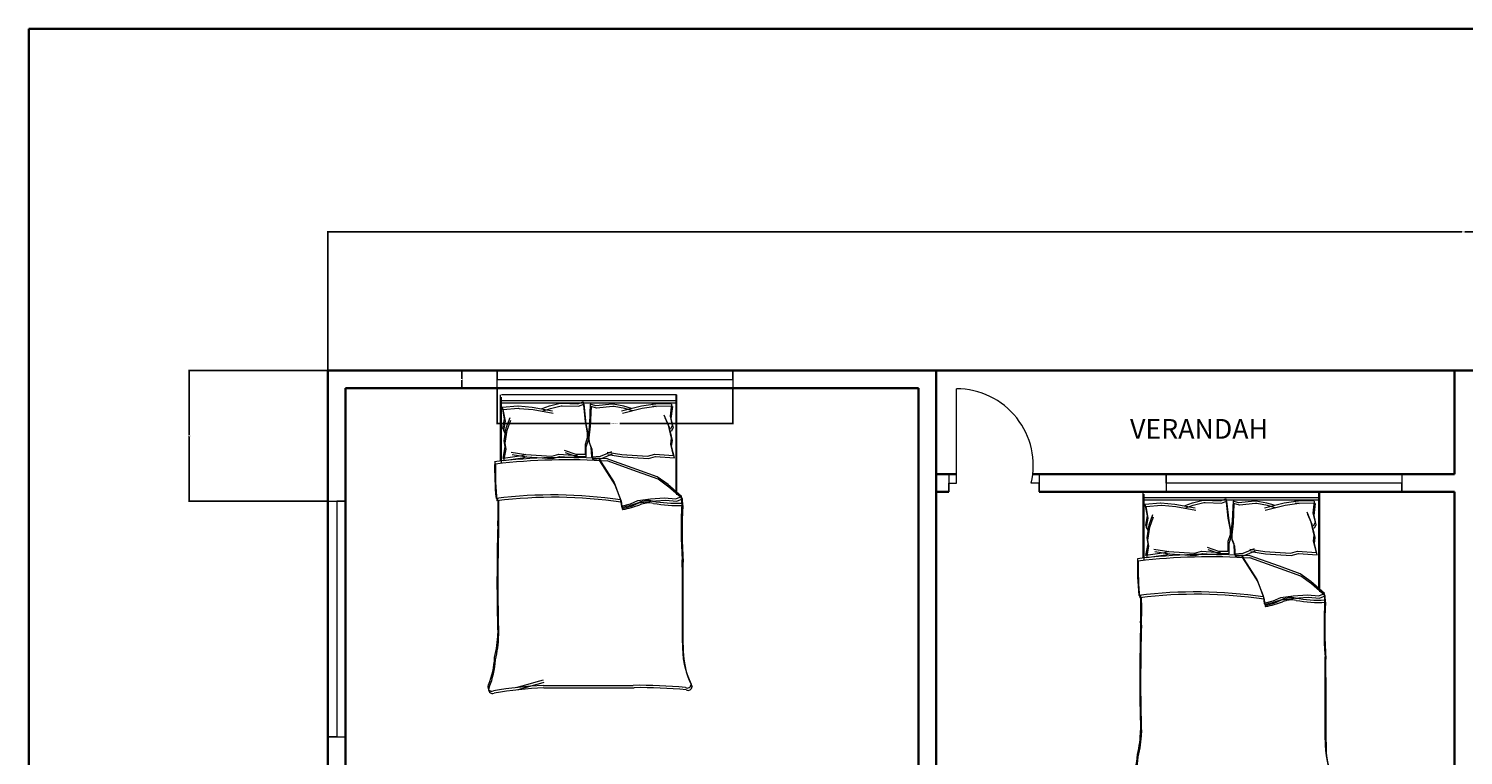
# Model space of a CAD drawing. Units: inches. Extents: x 2234 to 3001, y 1541 to 2386.
# Tile 7 of 12: x 2234 to 2599, y 2201 to 2386. Entities that reach past the tile are written whole.
import ezdxf

# ---------------------------------------------------------------- set-up
doc = ezdxf.new("R2010")
doc.units = ezdxf.units.IN
for name, color, linetype, lineweight in [('A-ANNO-DIMS', 2, 'Continuous', 18), ('A-ANNO-TTLB', 7, 'Continuous', 35), ('A-AREA-IDEN', 7, 'Continuous', 18), ('A-DOOR', 3, 'Continuous', 18), ('A-FURN', 9, 'Continuous', 13), ('A-GLAZ', 4, 'Continuous', 18), ('A-WALL', 7, 'Continuous', 35)]:
    doc.layers.add(name, color=color, linetype=linetype, lineweight=lineweight)
doc.styles.get("Standard").update_dxf_attribs({"font": 'arial.ttf'})
doc.dimstyles.get("Standard").update_dxf_attribs({"dimtxt": 0.18, "dimasz": 0.18, "dimexe": 0.18, "dimexo": 0.0625, "dimgap": 0.09, "dimtad": 0, "dimtih": 1, "dimtoh": 1, "dimdec": 4, "dimzin": 0, "dimdsep": 46, "dimtxsty": 'Standard', "dimcen": 0.09, "dimadec": 0, "dimazin": 0, "dimtfac": 1, "dimtdec": 4, "dimtofl": 0, "dimtmove": 0, "dimatfit": 3, "dimfxl": 1, "dimtolj": 1, "dimtzin": 0, "dimarcsym": 0})

# ---------------------------------------------------------------- blocks, each defined once
blk = doc.blocks.new('WIN-60-A')
for p, q in [((0, 60), (4.5, 60)), ((4.5, 60), (2.25, 60)), ((2.25, 60), (2.25, 0)), ((2.25, 0), (0, 0)), ((0, 0), (4.5, 0))]:
    blk.add_line(p, q)
blk = doc.blocks.new('WIN-60-B')
for p, q in [((0, 60), (4.5, 60)), ((4.5, 60), (2.25, 60)), ((2.25, 60), (2.25, 0)), ((4.5, 0), (0, 0)), ((2.25, 0), (4.5, 0))]:
    blk.add_line(p, q)
blk = doc.blocks.new('BED-DOUBLE-A')
for p, q in [((3.24, 59.14), (3.24, 76.05)), ((3.24, 59.14), (3.24, 76.05)), ((3.24, 74.62), (47.87, 74.62)), ((3.24, 74.62), (47.87, 74.62)), ((48.08, 76.05), (3.46, 76.05)), ((3.46, 58.54), (3.46, 75.45)), ((3.46, 58.54), (3.46, 75.45)), ((3.46, 74.02), (48.08, 74.02)), ((3.46, 74.02), (48.08, 74.02)), ((3.64, 72.93), (7.64, 73.24)), ((3.64, 72.93), (7.64, 73.24)), ((7.64, 73.24), (7.74, 73.22)), ((7.64, 73.24), (7.74, 73.22)), ((7.74, 73.22), (11.31, 72.95)), ((7.74, 73.22), (11.31, 72.95)), ((13.87, 72.55), (15.76, 73.22)), ((13.87, 72.55), (15.76, 73.22)), ((15.76, 73.22), (18.46, 73.9)), ((15.76, 73.22), (18.46, 73.9)), ((15.97, 72.62), (18.67, 73.3)), ((15.97, 72.62), (18.67, 73.3)), ((18.46, 73.9), (18.76, 73.9)), ((18.46, 73.9), (18.76, 73.9)), ((18.67, 73.3), (18.97, 73.3)), ((18.67, 73.3), (18.97, 73.3)), ((18.76, 73.9), (22.91, 73.76)), ((18.76, 73.9), (22.91, 73.76)), ((18.97, 73.3), (23.12, 73.16)), ((18.97, 73.3), (23.12, 73.16)), ((22.91, 73.76), (24.26, 74.3)), ((22.91, 73.76), (24.26, 74.3)), ((23.12, 73.16), (24.47, 73.7)), ((23.12, 73.16), (24.47, 73.7)), ((24.26, 74.3), (24.8, 69.31)), ((24.26, 74.3), (24.8, 69.31)), ((24.47, 73.7), (25.01, 68.71)), ((24.47, 73.7), (25.01, 68.71)), ((26.12, 73.72), (25.9, 68.7)), ((26.12, 73.72), (25.9, 68.7)), ((26.34, 73.12), (26.11, 68.1)), ((26.34, 73.12), (26.11, 68.1)), ((27.5, 73.27), (26.12, 73.72)), ((27.5, 73.27), (26.12, 73.72)), ((27.72, 72.67), (26.34, 73.12)), ((27.72, 72.67), (26.34, 73.12)), ((31.64, 73.66), (27.5, 73.27)), ((31.64, 73.66), (27.5, 73.27)), ((31.94, 73.68), (31.64, 73.66)), ((31.94, 73.68), (31.64, 73.66)), ((34.67, 73.17), (31.94, 73.68)), ((34.67, 73.17), (31.94, 73.68)), ((39.14, 73.18), (34.08, 71.92)), ((39.14, 73.18), (34.08, 71.92)), ((36.6, 72.62), (34.67, 73.17)), ((36.6, 72.62), (34.67, 73.17)), ((42.68, 73.67), (39.14, 73.18)), ((42.68, 73.67), (39.14, 73.18)), ((46.79, 73.66), (41.75, 73.75)), ((41.75, 73.75), (42.68, 73.67)), ((46.79, 73.66), (41.75, 73.75)), ((41.75, 73.75), (42.68, 73.67)), ((47.01, 73.06), (41.96, 73.15)), ((41.96, 73.15), (42.9, 73.08)), ((47, 73.06), (41.96, 73.15)), ((41.96, 73.15), (42.9, 73.08)), ((46.79, 73.66), (46.44, 70.66)), ((46.79, 73.66), (46.44, 70.66)), ((47.87, 76.05), (47.87, 51.2)), ((47.87, 76.05), (47.87, 51.2)), ((48.08, 76.05), (48.08, 75.45)), ((48.08, 75.45), (48.08, 50.6)), ((48.08, 75.45), (48.08, 50.6)), ((3.64, 72.95), (4.18, 69.98)), ((3.64, 72.95), (4.18, 69.98)), ((4.18, 69.98), (3.77, 67.55)), ((4.18, 69.98), (3.77, 67.55)), ((3.85, 72.33), (7.85, 72.64)), ((3.85, 72.33), (7.85, 72.64)), ((3.85, 72.35), (4.39, 69.38)), ((3.85, 72.35), (4.39, 69.38)), ((4.72, 67.69), (5.66, 70.25)), ((4.72, 67.69), (5.66, 70.25)), ((4.93, 67.09), (5.87, 69.65)), ((4.93, 67.09), (5.87, 69.65)), ((7.85, 72.64), (7.95, 72.62)), ((7.85, 72.64), (7.95, 72.62)), ((7.95, 72.62), (11.52, 72.35)), ((7.95, 72.62), (11.52, 72.35)), ((11.31, 72.95), (16.44, 72.01)), ((11.31, 72.95), (16.44, 72.01)), ((11.52, 72.35), (16.65, 71.41)), ((11.52, 72.35), (16.65, 71.41)), ((14.08, 71.95), (15.97, 72.62)), ((14.08, 71.95), (15.97, 72.62)), ((31.85, 73.06), (27.72, 72.67)), ((31.85, 73.06), (27.72, 72.67)), ((32.15, 73.08), (31.85, 73.06)), ((32.15, 73.08), (31.85, 73.06)), ((34.89, 72.58), (32.15, 73.08)), ((34.89, 72.58), (32.15, 73.08)), ((39.35, 72.58), (34.29, 71.32)), ((39.35, 72.58), (34.29, 71.32)), ((36.82, 72.02), (34.89, 72.58)), ((36.82, 72.02), (34.89, 72.58)), ((42.9, 73.08), (39.35, 72.58)), ((42.9, 73.08), (39.35, 72.58)), ((46.04, 68.34), (44.94, 70.84)), ((46.04, 68.34), (44.94, 70.84)), ((46.26, 67.74), (45.15, 70.24)), ((46.26, 67.74), (45.15, 70.24)), ((46.44, 70.66), (46.99, 68.26)), ((46.44, 70.66), (46.99, 68.26)), ((47.01, 73.06), (46.65, 70.07)), ((47, 73.06), (46.65, 70.07)), ((46.65, 70.07), (47.21, 67.66)), ((46.65, 70.07), (47.21, 67.66)), ((3.77, 67.55), (4.31, 66.61)), ((3.77, 67.55), (4.31, 66.61)), ((4.39, 69.38), (3.98, 66.95)), ((4.39, 69.38), (3.98, 66.95)), ((3.98, 66.95), (4.52, 66.01)), ((3.98, 66.95), (4.52, 66.01)), ((4.18, 64.31), (4.72, 67.69)), ((4.18, 64.31), (4.72, 67.69)), ((4.39, 63.71), (4.93, 67.09)), ((4.39, 63.71), (4.93, 67.09)), ((24.8, 69.31), (25.34, 66.34)), ((24.8, 69.31), (25.34, 66.34)), ((25.01, 68.71), (25.55, 65.74)), ((25.01, 68.71), (25.55, 65.74)), ((25.34, 66.34), (25.34, 65.12)), ((25.34, 66.34), (25.34, 65.12)), ((25.9, 68.7), (25.54, 65.7)), ((25.9, 68.7), (25.54, 65.7)), ((26.11, 68.1), (25.76, 65.11)), ((26.11, 68.1), (25.76, 65.11)), ((46.79, 65), (46.04, 68.34)), ((46.79, 65), (46.04, 68.34)), ((47.01, 64.41), (46.26, 67.74)), ((47, 64.41), (46.26, 67.74)), ((46.99, 68.26), (46.51, 67.28)), ((46.99, 68.26), (46.51, 67.28)), ((47.21, 67.66), (46.73, 66.69)), ((47.21, 67.66), (46.73, 66.69)), ((3.91, 59.86), (4.45, 62.83)), ((3.91, 59.86), (4.45, 62.83)), ((4.12, 59.26), (4.66, 62.23)), ((4.12, 59.26), (4.66, 62.23)), ((4.45, 62.83), (4.18, 64.31)), ((4.45, 62.83), (4.18, 64.31)), ((4.66, 62.23), (4.39, 63.71)), ((4.66, 62.23), (4.39, 63.71)), ((25.34, 65.12), (24.8, 63.37)), ((25.34, 65.12), (24.8, 63.37)), ((24.8, 63.37), (24.8, 60.86)), ((24.8, 63.37), (24.8, 60.86)), ((25.55, 64.52), (25.01, 62.77)), ((25.55, 64.52), (25.01, 62.77)), ((25.01, 62.77), (25.01, 60.27)), ((25.01, 62.77), (25.01, 60.27)), ((25.54, 65.7), (25.62, 64.49)), ((25.54, 65.7), (25.62, 64.49)), ((25.55, 65.74), (25.55, 64.52)), ((25.55, 65.74), (25.55, 64.52)), ((25.62, 64.49), (26.27, 62.77)), ((25.62, 64.49), (26.27, 62.77)), ((25.76, 65.11), (25.83, 63.89)), ((25.76, 65.11), (25.83, 63.89)), ((25.83, 63.89), (26.48, 62.18)), ((25.83, 63.89), (26.48, 62.18)), ((26.27, 62.77), (26.42, 60.27)), ((26.27, 62.77), (26.42, 60.27)), ((26.48, 62.18), (26.64, 59.68)), ((26.48, 62.18), (26.64, 59.68)), ((46.61, 63.5), (46.79, 65)), ((47.34, 60.57), (46.61, 63.5)), ((46.62, 63.5), (46.79, 65)), ((47.34, 60.57), (46.62, 63.5)), ((46.83, 62.91), (47.01, 64.41)), ((46.83, 62.91), (47, 64.41)), ((47.55, 59.98), (46.83, 62.91)), ((47.55, 59.98), (46.83, 62.91)), ((8.67, 60.53), (3.91, 59.86)), ((8.67, 60.53), (3.91, 59.86)), ((8.88, 59.93), (4.12, 59.26)), ((8.88, 59.93), (4.12, 59.26)), ((5.96, 61.45), (9.72, 60.83)), ((5.96, 61.45), (9.72, 60.83)), ((6.17, 60.86), (9.94, 60.24)), ((6.17, 60.86), (9.94, 60.24)), ((9.72, 60.83), (8.67, 60.53)), ((9.72, 60.83), (8.67, 60.53)), ((9.94, 60.24), (8.88, 59.93)), ((9.94, 60.24), (8.88, 59.93)), ((9.72, 60.83), (16.27, 60.43)), ((9.72, 60.83), (16.27, 60.43)), ((9.94, 60.24), (16.48, 59.83)), ((9.94, 60.24), (16.48, 59.83)), ((16.27, 60.43), (18.1, 60.95)), ((16.27, 60.43), (18.1, 60.95)), ((16.48, 59.83), (18.31, 60.35)), ((16.48, 59.83), (18.31, 60.35)), ((18.1, 60.95), (22.89, 60.57)), ((18.1, 60.95), (22.89, 60.57)), ((18.31, 60.35), (23.1, 59.98)), ((18.31, 60.35), (23.1, 59.98)), ((22.51, 60.86), (19.57, 61.88)), ((22.51, 60.86), (19.57, 61.88)), ((22.72, 60.27), (19.78, 61.28)), ((22.72, 60.27), (19.78, 61.28)), ((24.8, 60.86), (22.51, 60.86)), ((24.8, 60.86), (22.51, 60.86)), ((25.01, 60.27), (22.72, 60.27)), ((25.01, 60.27), (22.72, 60.27)), ((26.42, 60.27), (28.71, 60.42)), ((26.42, 60.27), (28.71, 60.42)), ((26.64, 59.68), (28.93, 59.82)), ((26.64, 59.68), (28.93, 59.82)), ((28.25, 59.82), (32.17, 53.75)), ((28.25, 59.82), (32.17, 53.75)), ((28.47, 59.22), (32.38, 53.16)), ((28.47, 59.22), (32.38, 53.16)), ((28.71, 60.42), (31.58, 61.62)), ((28.71, 60.42), (31.58, 61.62)), ((28.93, 59.82), (31.79, 61.02)), ((28.93, 59.82), (31.79, 61.02)), ((37.95, 57.08), (30.17, 59.82)), ((37.95, 57.08), (30.17, 59.82)), ((38.16, 56.48), (30.38, 59.22)), ((38.16, 56.48), (30.38, 59.22)), ((30.41, 61.45), (34.17, 60.83)), ((30.41, 61.45), (34.17, 60.83)), ((30.62, 60.86), (34.38, 60.24)), ((30.62, 60.86), (34.38, 60.24)), ((34.17, 60.83), (40.72, 60.43)), ((34.17, 60.83), (40.72, 60.43)), ((34.38, 60.24), (40.93, 59.83)), ((34.38, 60.24), (40.93, 59.83)), ((40.72, 60.43), (42.55, 60.95)), ((40.72, 60.43), (42.55, 60.95)), ((40.93, 59.83), (42.76, 60.35)), ((40.93, 59.83), (42.76, 60.35)), ((42.55, 60.95), (47.34, 60.57)), ((42.55, 60.95), (47.34, 60.57)), ((42.76, 60.35), (47.55, 59.98)), ((42.76, 60.35), (47.55, 59.98)), ((43.16, 55.2), (37.95, 57.08)), ((43.16, 55.2), (37.95, 57.08)), ((43.37, 54.6), (38.16, 56.48)), ((43.37, 54.6), (38.16, 56.48)), ((45.91, 53.18), (43.16, 55.2)), ((45.9, 53.18), (43.16, 55.2)), ((32.17, 53.75), (33.76, 49.56)), ((32.17, 53.75), (33.76, 49.56)), ((32.38, 53.16), (33.97, 48.97)), ((32.38, 53.16), (33.97, 48.97)), ((46.12, 52.58), (43.37, 54.6)), ((46.12, 52.58), (43.37, 54.6)), ((49.36, 50.14), (45.9, 53.18)), ((49.37, 50.14), (45.91, 53.18)), ((49.58, 49.54), (46.12, 52.58)), ((49.58, 49.54), (46.12, 52.58)), ((33.76, 49.56), (34.05, 47.68)), ((33.76, 49.56), (34.05, 47.68)), ((33.97, 48.97), (34.26, 47.09)), ((33.97, 48.97), (34.26, 47.09)), ((34.05, 47.68), (36.36, 48.26)), ((34.05, 47.68), (36.36, 48.26)), ((34.26, 47.09), (36.57, 47.66)), ((34.26, 47.09), (36.57, 47.66)), ((36.36, 48.26), (38.24, 49.13)), ((36.36, 48.26), (38.24, 49.13)), ((36.57, 47.66), (38.45, 48.53)), ((36.57, 47.66), (38.45, 48.53)), ((38.24, 49.13), (41.42, 49.56)), ((38.24, 49.13), (41.42, 49.56)), ((38.45, 48.53), (41.64, 48.97)), ((38.45, 48.53), (41.64, 48.97)), ((41.42, 49.56), (45.04, 49.85)), ((41.42, 49.56), (45.04, 49.85)), ((41.64, 48.97), (45.25, 49.25)), ((41.64, 48.97), (45.25, 49.25)), ((45.04, 49.85), (47.93, 49.56)), ((45.04, 49.85), (47.93, 49.56)), ((45.25, 49.25), (48.14, 48.97)), ((45.25, 49.25), (48.14, 48.97)), ((47.93, 49.56), (49.37, 50.14)), ((47.93, 49.56), (49.36, 50.14)), ((48.14, 48.97), (49.58, 49.54)), ((48.14, 48.97), (49.58, 49.54)), ((49.44, 48.51), (49.36, 50.14, 3.61)), ((49.44, 48.51), (49.37, 50.14, 3.61)), ((49.65, 47.91), (49.58, 49.54, 3.61)), ((49.65, 47.91), (49.58, 49.54, 3.61)), ((14.07, 2.05), (37.05, 2.05)), ((14.07, 2.05), (37.05, 2.05)), ((14.28, 1.46), (37.26, 1.46)), ((14.28, 1.46), (37.26, 1.46))]:
    blk.add_line(p, q)
for centre, radius, start, end in [((79.52, 57.28), 77.79, 178.7218, 185.604), ((79.52, 57.28), 77.79, 178.7218, 185.604), ((19.94, -93.94), 154.04, 86.0865, 96.7821), ((19.94, -93.94), 154.04, 86.0865, 96.7821), ((20.16, -94.54), 154.04, 86.0865, 96.7821), ((20.16, -94.54), 154.04, 86.0865, 96.7821), ((79.73, 56.69), 77.79, 178.7218, 185.604), ((79.73, 56.69), 77.79, 178.7218, 185.604), ((16.58, -69.91), 120.47, 81.7845, 96.9006), ((16.58, -69.91), 120.47, 81.7845, 96.9006), ((16.79, -70.51), 120.47, 81.7845, 96.9006), ((16.79, -70.51), 120.47, 81.7845, 96.9006), ((-156.22, 46.94), 158.84, 358.4762, 1.0082), ((-156.22, 46.94), 158.84, 358.4762, 1.0082), ((-156.01, 46.34), 158.84, 358.4762, 1.0082), ((-156.01, 46.34), 158.84, 358.4762, 1.0082), ((34.21, 47.63), 0.172, 160.2464, 271.1377), ((34.21, 47.63), 0.172, 160.2464, 271.1377), ((29.09, 74.66), 27.69, 280.6617, 289.8806), ((29.09, 74.66), 27.69, 280.6617, 289.8806), ((29.3, 74.07), 27.69, 280.6617, 289.8806), ((29.3, 74.07), 27.69, 280.6617, 289.8806), ((40.85, 43.3), 5.81, 78.6608, 113.7384), ((40.85, 43.3), 5.81, 78.6608, 113.7384), ((41.06, 42.71), 5.81, 78.6608, 113.7384), ((41.06, 42.71), 5.81, 78.6608, 113.7384), ((47.93, 82.26), 33.79, 259.8763, 272.5657), ((47.93, 82.26), 33.79, 259.8763, 272.5657), ((48.14, 81.67), 33.79, 259.8763, 272.5657), ((48.14, 81.67), 33.79, 259.8763, 272.5657), ((170.19, 42.14), 120.92, 176.9791, 183.8365), ((170.19, 42.14), 120.92, 176.9791, 183.8365), ((170.4, 41.54), 120.92, 176.9791, 183.8365), ((170.4, 41.54), 120.92, 176.9791, 183.8365), ((34.42, 47.03), 0.172, 160.2464, 271.1377), ((34.42, 47.03), 0.172, 160.2464, 271.1377), ((452.7, 28.79), 450.36, 178.2277, 181.7185), ((452.7, 28.79), 450.36, 178.2277, 181.7185), ((452.91, 28.19), 450.36, 178.2277, 181.7185), ((452.91, 28.19), 450.36, 178.2277, 181.7185), ((-4210.02, 12.72), 4259.62, 0.00217, 0.28689), ((-4210.02, 12.72), 4259.62, 0.00217, 0.28689), ((-4209.81, 12.12), 4259.62, 0.00217, 0.28689), ((-4209.81, 12.12), 4259.62, 0.00217, 0.28689), ((-25.12, 15.81), 27.67, 346.0648, 358.9113), ((-25.12, 15.81), 27.67, 346.0648, 358.9113), ((-24.9, 15.21), 27.67, 346.0648, 358.9113), ((-24.9, 15.21), 27.67, 346.0648, 358.9113), ((71.11, 11.93), 21.54, 177.4714, 206.4681), ((71.11, 11.93), 21.54, 177.4714, 206.4681), ((71.32, 11.33), 21.54, 177.4714, 206.4681), ((71.32, 11.33), 21.54, 177.4714, 206.4681), ((-20.22, 10.43), 22, 337.9751, 356.652), ((-20.22, 10.43), 22, 337.9751, 356.652), ((-20.01, 9.83), 22, 337.9751, 356.652), ((-20.01, 9.83), 22, 337.9751, 356.652), ((1.02, 1.61), 1.02, 146.1736, 293.4781), ((1.02, 1.61), 1.02, 146.1736, 293.4781), ((1.23, 1.01), 1.02, 146.1736, 293.4781), ((1.23, 1.01), 1.02, 146.1736, 293.4781), ((20.01, -111.48), 113.69, 92.9958, 99.4091), ((20.01, -111.48), 113.69, 92.9958, 99.4091), ((20.22, -112.08), 113.69, 92.9958, 99.4091), ((20.22, -112.08), 113.69, 92.9958, 99.4091), ((-16.08, 98.19), 99.41, 283.3832, 287.7053), ((-16.08, 98.19), 99.41, 283.3832, 287.7053), ((-15.87, 97.59), 99.41, 283.3832, 287.7053), ((-15.87, 97.59), 99.41, 283.3832, 287.7053), ((38.43, -122.16), 124.23, 84.4998, 90.6351), ((38.43, -122.16), 124.23, 84.4998, 90.6351), ((38.64, -122.76), 124.23, 84.4998, 90.6351), ((38.64, -122.76), 124.23, 84.4998, 90.6351), ((50.81, 2.4), 1.03, 242.6588, 356.02), ((50.8, 2.4), 1.03, 242.6588, 356.02), ((51.02, 1.81), 1.03, 242.6588, 356.02), ((51.02, 1.81), 1.03, 242.6588, 356.02)]:
    blk.add_arc(centre, radius, start, end)
blk = doc.blocks.new('*D27')
at = {"layer": 'A-ANNO-DIMS', "color": 0, "lineweight": -2, "transparency": 16777216}
for p, q in [((2352.89, 2294.05), (2352.89, 2284.93)), ((2412.89, 2294.05), (2412.89, 2284.93)), ((2353.07, 2285.11), (2381.65, 2285.11)), ((2412.71, 2285.11), (2384.12, 2285.11))]:
    blk.add_line(p, q, dxfattribs=at)
at = {"layer": 'A-ANNO-DIMS', "color": 0, "transparency": 16777216}
for points in [[(2353.07, 2285.14), (2353.07, 2285.08), (2352.89, 2285.11)], [(2412.71, 2285.14), (2412.71, 2285.08), (2412.89, 2285.11)]]:
    blk.add_solid(points, dxfattribs=at)
at = {"layer": 'Defpoints', "color": 0, "transparency": 16777216}
for p in [(2352.89, 2294.11), (2412.89, 2294.11), (2352.89, 2285.11)]:
    blk.add_point(p, dxfattribs=at)
at = {"layer": 'A-ANNO-DIMS', "color": 0, "transparency": 16777216, "insert": (2382.89, 2285.11), "char_height": 0.18, "attachment_point": 5}
blk.add_mtext('\\A1;WINDOW B 60 TYP.', dxfattribs=at)
blk = doc.blocks.new('*D28')
at = {"layer": 'A-ANNO-DIMS', "color": 0, "lineweight": -2, "transparency": 16777216}
for p, q in [((2352.82, 2298.61), (2343.71, 2298.61)), ((2343.89, 2298.43), (2343.89, 2296.54)), ((2343.89, 2294.29), (2343.89, 2296.18)), ((2352.82, 2294.11), (2343.71, 2294.11))]:
    blk.add_line(p, q, dxfattribs=at)
at = {"layer": 'A-ANNO-DIMS', "color": 0, "transparency": 16777216}
for points in [[(2343.86, 2298.43), (2343.92, 2298.43), (2343.89, 2298.61)], [(2343.86, 2294.29), (2343.92, 2294.29), (2343.89, 2294.11)]]:
    blk.add_solid(points, dxfattribs=at)
at = {"layer": 'Defpoints', "color": 0, "transparency": 16777216}
for p in [(2343.89, 2298.61), (2352.89, 2298.61), (2352.89, 2294.11)]:
    blk.add_point(p, dxfattribs=at)
at = {"layer": 'A-ANNO-DIMS', "color": 0, "transparency": 16777216, "insert": (2343.89, 2296.36), "char_height": 0.18, "attachment_point": 5}
blk.add_mtext('\\A1;5 TYP.', dxfattribs=at)
blk = doc.blocks.new('*D61')
at = {"layer": 'A-ANNO-DIMS', "color": 0, "lineweight": -2, "transparency": 16777216}
for p, q in [((2309.75, 2298.67), (2309.75, 2334.14)), ((2309.93, 2333.96), (2598.61, 2333.96)), ((2888.07, 2333.96), (2599.4, 2333.96)), ((2888.25, 2298.67), (2888.25, 2334.14))]:
    blk.add_line(p, q, dxfattribs=at)
at = {"layer": 'A-ANNO-DIMS', "color": 0, "transparency": 16777216}
for points in [[(2309.93, 2333.99), (2309.93, 2333.93), (2309.75, 2333.96)], [(2888.07, 2333.99), (2888.07, 2333.93), (2888.25, 2333.96)]]:
    blk.add_solid(points, dxfattribs=at)
at = {"layer": 'Defpoints', "color": 0, "transparency": 16777216}
for p in [(2888.25, 2333.96), (2309.75, 2298.61), (2888.25, 2298.61)]:
    blk.add_point(p, dxfattribs=at)
at = {"layer": 'A-ANNO-DIMS', "color": 0, "transparency": 16777216, "insert": (2599, 2333.96), "char_height": 0.18, "attachment_point": 5}
blk.add_mtext('\\A1;578.5', dxfattribs=at)
blk = doc.blocks.new('*D70')
at = {"layer": 'A-ANNO-DIMS', "color": 0, "lineweight": -2, "transparency": 16777216}
for p, q in [((2309.69, 2298.61), (2274.22, 2298.61)), ((2274.4, 2298.43), (2274.4, 2282.15)), ((2274.4, 2265.51), (2274.4, 2281.79)), ((2309.69, 2265.33), (2274.22, 2265.33))]:
    blk.add_line(p, q, dxfattribs=at)
at = {"layer": 'A-ANNO-DIMS', "color": 0, "transparency": 16777216}
for points in [[(2274.37, 2298.43), (2274.43, 2298.43), (2274.4, 2298.61)], [(2274.37, 2265.51), (2274.43, 2265.51), (2274.4, 2265.33)]]:
    blk.add_solid(points, dxfattribs=at)
at = {"layer": 'Defpoints', "color": 0, "transparency": 16777216}
for p in [(2274.4, 2298.61), (2309.75, 2298.61), (2309.75, 2265.33)]:
    blk.add_point(p, dxfattribs=at)
at = {"layer": 'A-ANNO-DIMS', "color": 0, "transparency": 16777216, "insert": (2274.4, 2281.97), "char_height": 0.18, "attachment_point": 5}
blk.add_mtext('\\A1;33.28', dxfattribs=at)

msp = doc.modelspace()

# ---------------------------------------------------------------- linework, layer by layer
at = {"layer": 'A-ANNO-TTLB'}
msp.add_lwpolyline([(2233.5367, 2385.7012), (3001.3383, 2385.7012), (3001.3383, 1541.435), (2233.5367, 1541.435)], close=True, dxfattribs=at)
at = {"layer": 'A-DOOR'}
for p, q in [((2469.9199, 2269.9685), (2469.9199, 2293.9685)), ((2467.9199, 2272.2185), (2467.9199, 2267.7185)), ((2467.9199, 2267.7185), (2467.9199, 2269.9685)), ((2467.9199, 2269.9685), (2469.9199, 2269.9685)), ((2490.9272, 2269.9685), (2488.9272, 2269.9685)), ((2490.9272, 2272.2185), (2490.9272, 2267.7185)), ((2490.9272, 2267.7185), (2490.9272, 2269.9685))]:
    msp.add_line(p, q, dxfattribs=at)
msp.add_arc((2469.9199, 2274.4419), 19.5266, 346.756467, 90, dxfattribs=at)
at = {"layer": 'A-GLAZ'}
for p, q in [((2523.3188, 2272.2185), (2523.3188, 2272.2185)), ((2314.2534, 2265.3327), (2314.2534, 2265.3327))]:
    msp.add_line(p, q, dxfattribs=at)
at = {"layer": 'A-WALL'}
for p, q in [((2309.7534, 2298.611), (2309.7534, 1702.111)), ((2309.7534, 2298.611), (2464.7534, 2298.611)), ((2464.7534, 2298.611), (2464.7534, 2157.611)), ((2464.7534, 2298.611), (2733.2534, 2298.611)), ((2596.7534, 2298.611), (2596.7534, 2272.2185)), ((2596.7534, 2298.611), (2601.2534, 2298.611)), ((2314.2534, 2294.111), (2460.2534, 2294.111)), ((2314.2534, 2294.111), (2314.2534, 2162.111)), ((2460.2534, 2294.111), (2460.2534, 2162.111)), ((2464.7534, 2258.111), (2464.7534, 2282.111)), ((2596.7534, 2277.611), (2596.7534, 2272.2185)), ((2464.7534, 2272.2185), (2469.9199, 2272.2185)), ((2489.3195, 2272.2185), (2596.7534, 2272.2185)), ((2464.7534, 2267.7185), (2467.9199, 2267.7185)), ((2490.9272, 2267.7185), (2596.7534, 2267.7185)), ((2596.7534, 2267.7185), (2596.7534, 2150.111))]:
    msp.add_line(p, q, dxfattribs=at)

# ---------------------------------------------------------------- block references
at = {"layer": 'A-FURN'}
for p in [(2350.494, 2216.374), (2514.2466, 2191.6708)]:
    msp.add_blockref('BED-DOUBLE-A', p, dxfattribs=at)
at = {"layer": 'A-GLAZ'}
for name, p, rotation in [('WIN-60-B', (2412.8876, 2294.1106), 90), ('WIN-60-A', (2523.3192, 2272.219), 270)]:
    msp.add_blockref(name, p, dxfattribs=dict(at, rotation=rotation))
msp.add_blockref('WIN-60-A', (2309.753, 2205.333), dxfattribs=at)

# ---------------------------------------------------------------- texts
at = {"layer": 'A-AREA-IDEN', "insert": (2514.102, 2286.2718), "char_height": 5, "attachment_point": 1}
msp.add_mtext_dynamic_manual_height_columns('VERANDAH', width=107.840646, gutter_width=12.5, heights=[0], dxfattribs=at)

# ---------------------------------------------------------------- dimensions: what is measured, and where the dimension line sits
at = {"layer": 'A-ANNO-DIMS'}
dim = msp.add_linear_dim(base=(2888.2534, 2333.961), p1=(2309.7534, 2298.611), p2=(2888.2534, 2298.611), dimstyle='Standard', override={"dimdec": 1, "dimlfac": 1, "dimrnd": 0, "dimzin": 0, "dimdsep": 46, "dimlunit": 2}, dxfattribs=at)
dim.commit()
dim.dimension.update_dxf_attribs({"geometry": '*D61', "text_midpoint": (2599.0034, 2333.961)})
dim = msp.add_linear_dim(base=(2274.4034, 2298.611), p1=(2309.7534, 2265.3327), p2=(2309.7534, 2298.611), angle=90, dimstyle='Standard', override={"dimdec": 2, "dimlfac": 1, "dimrnd": 0, "dimzin": 0, "dimdsep": 46, "dimlunit": 2}, dxfattribs=at)
dim.commit()
dim.dimension.update_dxf_attribs({"geometry": '*D70', "text_midpoint": (2274.4034, 2281.9719)})
for base, p1, p2, angle, text, picture, middle in [((2343.8872920061, 2298.6110170859), (2352.8872920061, 2294.1110170859), (2352.8872920061, 2298.6110170859), 90, '<> TYP.', '*D28', (2343.8872920061, 2296.3610170859)), ((2352.8873, 2285.111), (2412.8873, 2294.111), (2352.8873, 2294.111), 180, 'WINDOW B <> TYP.', '*D27', (2382.8873, 2285.111))]:
    dim = msp.add_linear_dim(base=base, p1=p1, p2=p2, angle=angle, text=text, dimstyle='Standard', override={"dimdec": 0, "dimlfac": 1, "dimrnd": 0, "dimzin": 0, "dimdsep": 46, "dimlunit": 2}, dxfattribs=at)
    dim.commit()
    dim.dimension.update_dxf_attribs({"geometry": picture, "text_midpoint": middle})

doc.saveas('drawing.dxf')
